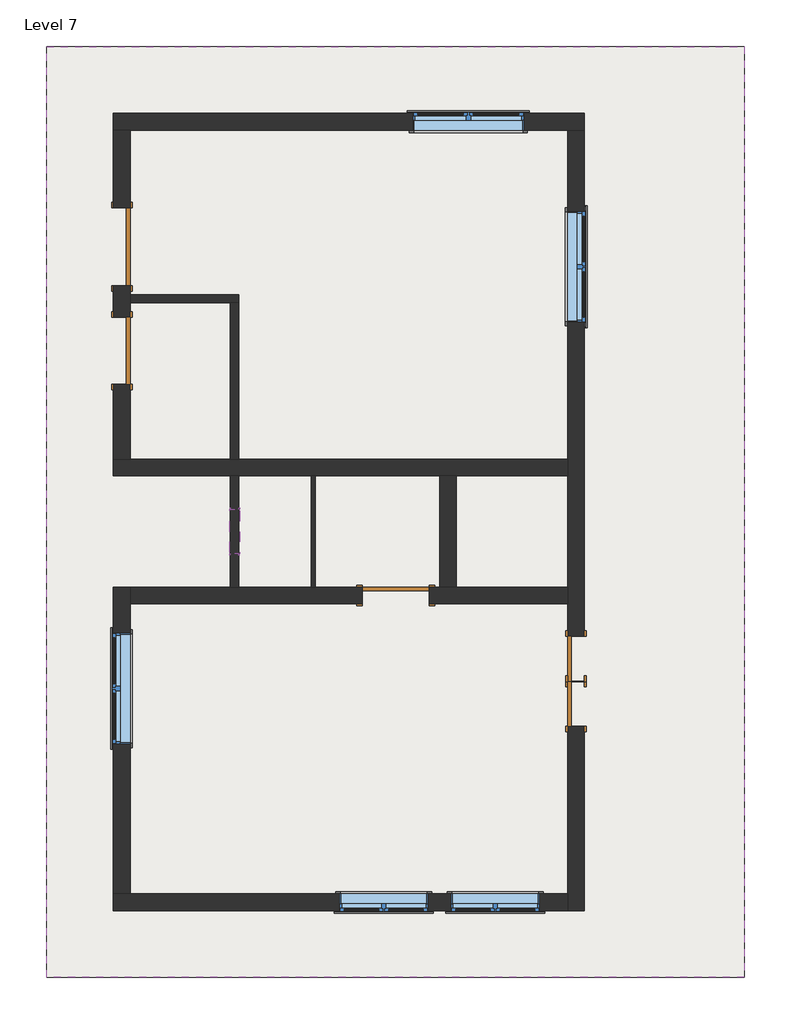
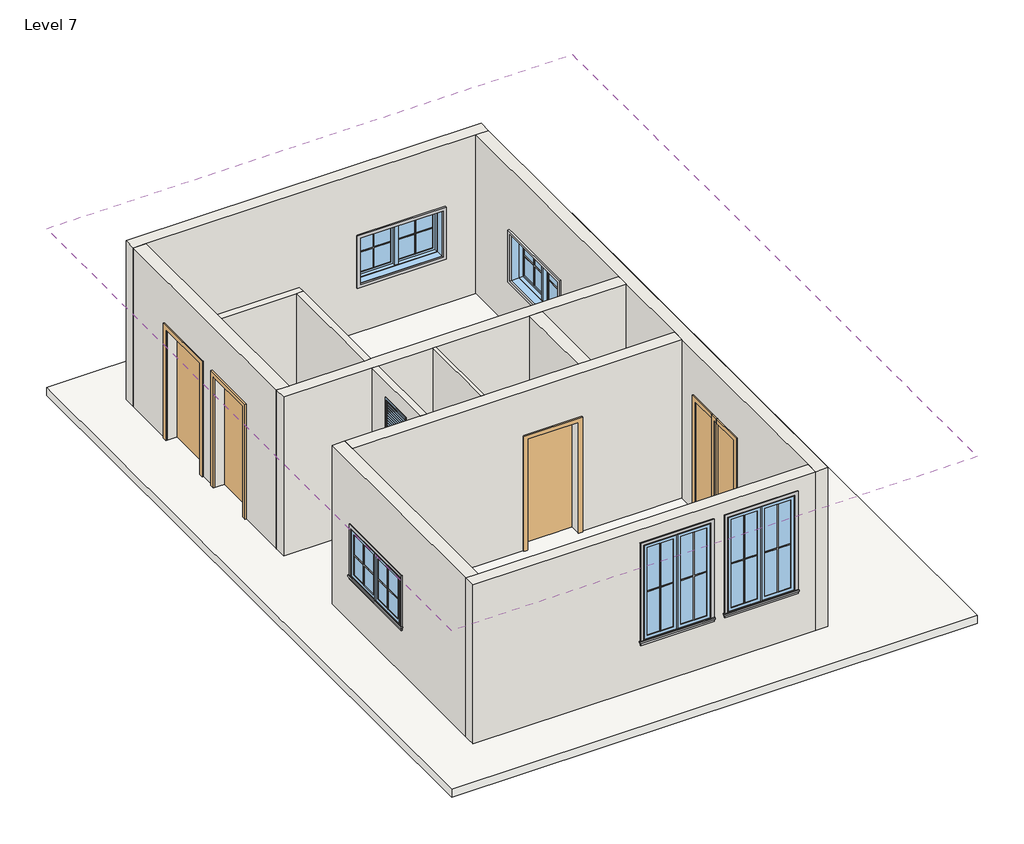
# One storey, incomplete: 20 proxies, 12 walls, 6 windows, 5 doors, 2 roofs.
"""IFC4 building model written with IfcOpenShell, lengths in millimetres."""

from ifc_helpers import new_model, si_unit, frame, origin, place, context, project, spatial, polyline, outline, extrude, faceted_brep, transform, mapped, element, save
from components import muntin_pattern_2x2_muntin_pattern_2x2_9352d081, muntin_pattern_2x2_muntin_pattern_2x2_5c2cbe28, muntin_pattern_2x2_muntin_pattern_2x2_2b4d9f72, muntin_pattern_2x2_muntin_pattern_2x2_ef995ed3, trim_window_exterior_flat_with_sill_979bde60, trim_window_exterior_flat_with_sill_b7e4d11c, trim_window_interior_flat_picture_frame_7883d11b, trim_window_interior_flat_picture_frame_936b8d2a, single_flush_door_2_0d3b4037, single_flush_door_2_4a3212df, door_a90ba1ad, door_0ca8825f, door_9d399b00, window_casement_double_c1d95f0f, window_casement_double_wall_4_6ca1769e, window_d39e7ecb

model = new_model("IFC4")

# Units and contexts
model_context = context("Model", 3, world=origin())
ifc_project = project(units=[si_unit("LENGTHUNIT", "METRE", prefix="MILLI")], contexts=[model_context])

# Site, building, storey
site = spatial("IfcSite", under=ifc_project)
building = spatial("IfcBuilding", under=site)
storey = spatial("IfcBuildingStorey", under=building, Name="Level 7", Elevation=16002.0)

# Proxies
placement = place(None, origin())
muntin_pattern_2x2_muntin_pattern_2x2_shape = muntin_pattern_2x2_muntin_pattern_2x2_9352d081(model_context)
element("IfcBuildingElementProxy", 1, Name="Muntin Pattern_2x2 : Muntin Pattern_2x2", ObjectType="Muntin Pattern_2x2 : Muntin Pattern_2x2", at=placement, inside=storey, context=model_context, shape_type="MappedRepresentation", body=[
    mapped(muntin_pattern_2x2_muntin_pattern_2x2_shape, transform((-4785.3510342, -2707.8617544, 16986.25), x_axis=(0.0, 1.0, 0.0), y_axis=(-1.0, 0.0, 0.0), z_axis=(0.0, 0.0, 1.0))),
])
element("IfcBuildingElementProxy", 2, Name="Muntin Pattern_2x2 : Muntin Pattern_2x2", ObjectType="Muntin Pattern_2x2 : Muntin Pattern_2x2", at=placement, inside=storey, context=model_context, shape_type="MappedRepresentation", body=[
    mapped(muntin_pattern_2x2_muntin_pattern_2x2_shape, transform((1634.4989658, 3816.7632456, 16986.25), x_axis=(0.0, -1.0, 0.0), y_axis=(1.0, 0.0, 0.0), z_axis=(0.0, 0.0, 1.0))),
])
element("IfcBuildingElementProxy", 3, Name="Muntin Pattern_2x2 : Muntin Pattern_2x2", ObjectType="Muntin Pattern_2x2 : Muntin Pattern_2x2", at=placement, inside=storey, context=model_context, shape_type="MappedRepresentation", body=[
    mapped(muntin_pattern_2x2_muntin_pattern_2x2_shape, transform((-322.8885342, 5523.3257456, 16986.25), x_axis=(1.0, 0.0, 0.0), y_axis=(0.0, 1.0, 0.0), z_axis=(0.0, 0.0, 1.0))),
])
muntin_pattern_2x2_muntin_pattern_2x2_2_shape = muntin_pattern_2x2_muntin_pattern_2x2_5c2cbe28(model_context)
element("IfcBuildingElementProxy", 4, Name="Muntin Pattern_2x2 : Muntin Pattern_2x2", ObjectType="Muntin Pattern_2x2 : Muntin Pattern_2x2", at=placement, inside=storey, context=model_context, shape_type="MappedRepresentation", body=[
    mapped(muntin_pattern_2x2_muntin_pattern_2x2_2_shape, transform((-4785.3510342, -1949.0367544, 16986.25), x_axis=(0.0, -1.0, 0.0), y_axis=(1.0, 0.0, 0.0), z_axis=(0.0, 0.0, 1.0))),
])
element("IfcBuildingElementProxy", 5, Name="Muntin Pattern_2x2 : Muntin Pattern_2x2", ObjectType="Muntin Pattern_2x2 : Muntin Pattern_2x2", at=placement, inside=storey, context=model_context, shape_type="MappedRepresentation", body=[
    mapped(muntin_pattern_2x2_muntin_pattern_2x2_2_shape, transform((1634.4989658, 3057.9382456, 16986.25), x_axis=(0.0, 1.0, 0.0), y_axis=(-1.0, 0.0, 0.0), z_axis=(0.0, 0.0, 1.0))),
])
element("IfcBuildingElementProxy", 6, Name="Muntin Pattern_2x2 : Muntin Pattern_2x2", ObjectType="Muntin Pattern_2x2 : Muntin Pattern_2x2", at=placement, inside=storey, context=model_context, shape_type="MappedRepresentation", body=[
    mapped(muntin_pattern_2x2_muntin_pattern_2x2_2_shape, transform((435.9364658, 5523.3257456, 16986.25), x_axis=(-1.0, 0.0, 0.0), y_axis=(0.0, -1.0, 0.0), z_axis=(0.0, 0.0, 1.0))),
])
muntin_pattern_2x2_muntin_pattern_2x2_3_shape = muntin_pattern_2x2_muntin_pattern_2x2_2b4d9f72(model_context)
element("IfcBuildingElementProxy", 7, Name="Muntin Pattern_2x2 : Muntin Pattern_2x2", ObjectType="Muntin Pattern_2x2 : Muntin Pattern_2x2", at=placement, inside=storey, context=model_context, shape_type="MappedRepresentation", body=[
    mapped(muntin_pattern_2x2_muntin_pattern_2x2_3_shape, transform((-795.9635342, -5354.2242544, 16986.25), x_axis=(-1.0, 0.0, 0.0), y_axis=(0.0, -1.0, 0.0), z_axis=(0.0, 0.0, 1.0))),
])
element("IfcBuildingElementProxy", 8, Name="Muntin Pattern_2x2 : Muntin Pattern_2x2", ObjectType="Muntin Pattern_2x2 : Muntin Pattern_2x2", at=placement, inside=storey, context=model_context, shape_type="MappedRepresentation", body=[
    mapped(muntin_pattern_2x2_muntin_pattern_2x2_3_shape, transform((728.0364658, -5354.2242544, 16986.25), x_axis=(-1.0, 0.0, 0.0), y_axis=(0.0, -1.0, 0.0), z_axis=(0.0, 0.0, 1.0))),
])
muntin_pattern_2x2_muntin_pattern_2x2_4_shape = muntin_pattern_2x2_muntin_pattern_2x2_ef995ed3(model_context)
element("IfcBuildingElementProxy", 9, Name="Muntin Pattern_2x2 : Muntin Pattern_2x2", ObjectType="Muntin Pattern_2x2 : Muntin Pattern_2x2", at=placement, inside=storey, context=model_context, shape_type="MappedRepresentation", body=[
    mapped(muntin_pattern_2x2_muntin_pattern_2x2_4_shape, transform((-1402.3885342, -5354.2242544, 16986.25), x_axis=(1.0, 0.0, 0.0), y_axis=(0.0, 1.0, 0.0), z_axis=(0.0, 0.0, 1.0))),
])
element("IfcBuildingElementProxy", 10, Name="Muntin Pattern_2x2 : Muntin Pattern_2x2", ObjectType="Muntin Pattern_2x2 : Muntin Pattern_2x2", at=placement, inside=storey, context=model_context, shape_type="MappedRepresentation", body=[
    mapped(muntin_pattern_2x2_muntin_pattern_2x2_4_shape, transform((121.6114658, -5354.2242544, 16986.25), x_axis=(1.0, 0.0, 0.0), y_axis=(0.0, 1.0, 0.0), z_axis=(0.0, 0.0, 1.0))),
])
trim_window_exterior_flat_with_sill_shape = trim_window_exterior_flat_with_sill_979bde60(model_context)
element("IfcBuildingElementProxy", 11, Name="Trim-Window-Exterior-Flat : with Sill", ObjectType="Trim-Window-Exterior-Flat : with Sill", at=placement, inside=storey, context=model_context, shape_type="MappedRepresentation", body=[
    mapped(trim_window_exterior_flat_with_sill_shape, transform((-4794.8760342, -2328.4492544, 17830.8), x_axis=(0.0, -1.0, 0.0), y_axis=(0.0, 0.0, 1.0), z_axis=(-1.0, 0.0, 0.0))),
])
element("IfcBuildingElementProxy", 12, Name="Trim-Window-Exterior-Flat : with Sill", ObjectType="Trim-Window-Exterior-Flat : with Sill", at=placement, inside=storey, context=model_context, shape_type="MappedRepresentation", body=[
    mapped(trim_window_exterior_flat_with_sill_shape, transform((1644.0239658, 3437.3507456, 17830.8), x_axis=(0.0, 1.0, 0.0), y_axis=(0.0, 0.0, 1.0), z_axis=(1.0, 0.0, 0.0))),
])
element("IfcBuildingElementProxy", 13, Name="Trim-Window-Exterior-Flat : with Sill", ObjectType="Trim-Window-Exterior-Flat : with Sill", at=placement, inside=storey, context=model_context, shape_type="MappedRepresentation", body=[
    mapped(trim_window_exterior_flat_with_sill_shape, transform((56.5239658, 5532.8507456, 17830.8), x_axis=(-1.0, 0.0, 0.0), y_axis=(0.0, 0.0, 1.0), z_axis=(0.0, 1.0, 0.0))),
])
trim_window_exterior_flat_with_sill_2_shape = trim_window_exterior_flat_with_sill_b7e4d11c(model_context)
element("IfcBuildingElementProxy", 14, Name="Trim-Window-Exterior-Flat : with Sill", ObjectType="Trim-Window-Exterior-Flat : with Sill", at=placement, inside=storey, context=model_context, shape_type="MappedRepresentation", body=[
    mapped(trim_window_exterior_flat_with_sill_2_shape, transform((-1099.1760342, -5363.7492544, 18745.2), x_axis=(1.0, 0.0, 0.0), y_axis=(0.0, 0.0, 1.0), z_axis=(0.0, -1.0, 0.0))),
])
element("IfcBuildingElementProxy", 15, Name="Trim-Window-Exterior-Flat : with Sill", ObjectType="Trim-Window-Exterior-Flat : with Sill", at=placement, inside=storey, context=model_context, shape_type="MappedRepresentation", body=[
    mapped(trim_window_exterior_flat_with_sill_2_shape, transform((424.8239658, -5363.7492544, 18745.2), x_axis=(1.0, 0.0, 0.0), y_axis=(0.0, 0.0, 1.0), z_axis=(0.0, -1.0, 0.0))),
])
trim_window_interior_flat_picture_frame_shape = trim_window_interior_flat_picture_frame_7883d11b(model_context)
element("IfcBuildingElementProxy", 16, Name="Trim-Window-Interior-Flat : Picture Frame", ObjectType="Trim-Window-Interior-Flat : Picture Frame", at=placement, inside=storey, context=model_context, shape_type="MappedRepresentation", body=[
    mapped(trim_window_interior_flat_picture_frame_shape, transform((-4566.2760342, -2328.4492544, 17830.8), x_axis=(0.0, 1.0, 0.0), y_axis=(0.0, 0.0, 1.0), z_axis=(1.0, 0.0, 0.0))),
])
element("IfcBuildingElementProxy", 17, Name="Trim-Window-Interior-Flat : Picture Frame", ObjectType="Trim-Window-Interior-Flat : Picture Frame", at=placement, inside=storey, context=model_context, shape_type="MappedRepresentation", body=[
    mapped(trim_window_interior_flat_picture_frame_shape, transform((1415.4239658, 3437.3507456, 17830.8), x_axis=(0.0, -1.0, 0.0), y_axis=(0.0, 0.0, 1.0), z_axis=(-1.0, 0.0, 0.0))),
])
element("IfcBuildingElementProxy", 18, Name="Trim-Window-Interior-Flat : Picture Frame", ObjectType="Trim-Window-Interior-Flat : Picture Frame", at=placement, inside=storey, context=model_context, shape_type="MappedRepresentation", body=[
    mapped(trim_window_interior_flat_picture_frame_shape, transform((56.5239658, 5304.2507456, 17830.8), x_axis=(1.0, 0.0, 0.0), y_axis=(0.0, 0.0, 1.0), z_axis=(0.0, -1.0, 0.0))),
])
trim_window_interior_flat_picture_frame_2_shape = trim_window_interior_flat_picture_frame_936b8d2a(model_context)
element("IfcBuildingElementProxy", 19, Name="Trim-Window-Interior-Flat : Picture Frame", ObjectType="Trim-Window-Interior-Flat : Picture Frame", at=placement, inside=storey, context=model_context, shape_type="MappedRepresentation", body=[
    mapped(trim_window_interior_flat_picture_frame_2_shape, transform((-1099.1760342, -5135.1492544, 18745.2), x_axis=(-1.0, 0.0, 0.0), y_axis=(0.0, 0.0, 1.0), z_axis=(0.0, 1.0, 0.0))),
])
element("IfcBuildingElementProxy", 20, Name="Trim-Window-Interior-Flat : Picture Frame", ObjectType="Trim-Window-Interior-Flat : Picture Frame", at=placement, inside=storey, context=model_context, shape_type="MappedRepresentation", body=[
    mapped(trim_window_interior_flat_picture_frame_2_shape, transform((424.8239658, -5135.1492544, 18745.2), x_axis=(-1.0, 0.0, 0.0), y_axis=(0.0, 0.0, 1.0), z_axis=(0.0, 1.0, 0.0))),
])

# Doors
single_flush_door_2_shape = single_flush_door_2_0d3b4037(model_context)
element("IfcDoor", 21, ObjectType="Single-Flush : door 2'", at=placement, inside=storey, context=model_context, shape_type="MappedRepresentation", body=[
    mapped(single_flush_door_2_shape, transform((1529.7239658, -1922.0492544, 16002.0), x_axis=(0.0, 1.0, 0.0), y_axis=(-1.0, 0.0, 0.0), z_axis=(0.0, 0.0, 1.0))),
])
single_flush_door_2_2_shape = single_flush_door_2_4a3212df(model_context)
element("IfcDoor", 22, ObjectType="Single-Flush : door 2'", at=placement, inside=storey, context=model_context, shape_type="MappedRepresentation", body=[
    mapped(single_flush_door_2_2_shape, transform((1529.7239658, -2537.9992544, 16002.0), x_axis=(0.0, -1.0, 0.0), y_axis=(1.0, 0.0, 0.0), z_axis=(0.0, 0.0, 1.0))),
])
door_shape = door_a90ba1ad(model_context)
element("IfcDoor", 23, ObjectType="Single-Flush : door 2'6\"", at=placement, inside=storey, context=model_context, shape_type="MappedRepresentation", body=[
    mapped(door_shape, transform((-4680.5760342, 2288.0007456, 16002.0), x_axis=(0.0, 1.0, 0.0), y_axis=(-1.0, 0.0, 0.0), z_axis=(0.0, 0.0, 1.0))),
])
door_2_shape = door_0ca8825f(model_context)
element("IfcDoor", 24, ObjectType="Single-Flush : door 2'6\"", at=placement, inside=storey, context=model_context, shape_type="MappedRepresentation", body=[
    mapped(door_2_shape, transform((-934.0760342, -1058.4492544, 16002.0), x_axis=(1.0, 0.0, 0.0), y_axis=(0.0, 1.0, 0.0), z_axis=(0.0, 0.0, 1.0))),
])
door_3_shape = door_9d399b00(model_context)
element("IfcDoor", 25, ObjectType="Single-Flush : door 3'6\"", at=placement, inside=storey, context=model_context, shape_type="MappedRepresentation", body=[
    mapped(door_3_shape, transform((-4680.5760342, 3710.4007456, 16002.0), x_axis=(0.0, -1.0, 0.0), y_axis=(1.0, 0.0, 0.0), z_axis=(0.0, 0.0, 1.0))),
])

# Roofs
element("IfcRoof", 26, ObjectType="roof 6\"", at=placement, inside=storey, context=model_context, shape_type="SweptSolid", body=[
    extrude(outline(polyline([(-5709.2760342, 6447.2507456), (3828.4239658, 6447.2507456), (3828.4239658, -6278.1492544), (-5709.2760342, -6278.1492544), (-5709.2760342, 6447.2507456)])), frame((0.0, 0.0, 15849.6), z_axis=(0.0, 0.0, 1.0), x_axis=(1.0, 0.0, 0.0)), (0.0, 0.0, 1.0), 152.4),
])
element("IfcRoof", 27, ObjectType="roof 6\"", at=placement, inside=storey, context=model_context, shape_type="SweptSolid", body=[
    extrude(outline(polyline([(-5709.2760342, 6447.2507456), (3828.4239658, 6447.2507456), (3828.4239658, -6278.1492544), (-5709.2760342, -6278.1492544), (-5709.2760342, 6447.2507456)])), frame((0.0, 0.0, 19050.0), z_axis=(0.0, 0.0, 1.0), x_axis=(1.0, 0.0, 0.0)), (0.0, 0.0, 1.0), 152.4),
])

# Walls
element("IfcWall", 28, ObjectType="wall 2\"", at=placement, inside=storey, context=model_context, shape_type="SweptSolid", body=[
    extrude(outline(polyline([(-2089.7760342, -944.1492544), (-2089.7760342, 579.8507456), (-2038.9760342, 579.8507456), (-2038.9760342, -944.1492544), (-2089.7760342, -944.1492544)])), frame((0.0, 0.0, 16002.0), z_axis=(0.0, 0.0, 1.0), x_axis=(1.0, 0.0, 0.0)), (0.0, 0.0, 1.0), 3048.0),
])
element("IfcWall", 29, ObjectType="wall 4.5\"", at=placement, inside=storey, context=model_context, shape_type="Brep", body=[
    faceted_brep([(-4566.2760342, 2942.0507456, 16002.0), (-3194.6760342, 2942.0507456, 16002.0), (-3080.3760342, 2942.0507456, 16002.0), (-3080.3760342, 2942.0507456, 19050.0), (-3194.6760342, 2942.0507456, 19050.0), (-4566.2760342, 2942.0507456, 19050.0), (-4566.2760342, 3056.3507456, 16002.0), (-4566.2760342, 3056.3507456, 19050.0), (-3080.3760342, 3056.3507456, 19050.0), (-3080.3760342, 3056.3507456, 16002.0)], [[[0, 1, 2, 3, 4, 5]], [[6, 7, 8, 9]], [[2, 1, 0, 6, 9]], [[0, 5, 7, 6]], [[3, 2, 9, 8]], [[5, 4, 3, 8, 7]]]),
])
element("IfcWall", 30, ObjectType="wall 4.5\"", at=placement, inside=storey, context=model_context, shape_type="SweptSolid", body=[
    extrude(outline(polyline([(-3194.6760342, 808.4507456), (-3194.6760342, 2942.0507456), (-3080.3760342, 2942.0507456), (-3080.3760342, 808.4507456), (-3194.6760342, 808.4507456)])), frame((0.0, 0.0, 16002.0), z_axis=(0.0, 0.0, 1.0), x_axis=(1.0, 0.0, 0.0)), (0.0, 0.0, 1.0), 3048.0),
])
element("IfcWall", 31, ObjectType="wall 4.5\"", at=placement, inside=storey, context=model_context, shape_type="SweptSolid", body=[
    extrude(outline(polyline([(579.8507456, 16002.0), (-944.1492544, 16002.0), (-944.1492544, 19050.0), (579.8507456, 19050.0), (579.8507456, 16002.0)]), holes=[polyline([(-486.9492544, 18745.2), (-486.9492544, 18135.6), (122.6507456, 18135.6), (122.6507456, 18745.2), (-486.9492544, 18745.2)])]), frame((-3194.6760342, 0.0, 0.0), z_axis=(1.0, 0.0, 0.0), x_axis=(0.0, 1.0, 0.0)), (0.0, 0.0, 1.0), 114.3),
])
element("IfcWall", 32, ObjectType="wall 9\"", at=placement, inside=storey, context=model_context, shape_type="Brep", body=[
    faceted_brep([(-4794.8760342, 5304.2507456, 16002.0), (-4566.2760342, 5304.2507456, 16002.0), (1415.4239658, 5304.2507456, 16002.0), (1644.0239658, 5304.2507456, 16002.0), (1644.0239658, 5304.2507456, 19050.0), (1415.4239658, 5304.2507456, 19050.0), (-4566.2760342, 5304.2507456, 19050.0), (-4794.8760342, 5304.2507456, 19050.0), (818.5239658, 5304.2507456, 17830.8), (818.5239658, 5304.2507456, 16916.4), (-705.4760342, 5304.2507456, 16916.4), (-705.4760342, 5304.2507456, 17830.8), (-4794.8760342, 5532.8507456, 16002.0), (-4794.8760342, 5532.8507456, 19050.0), (1644.0239658, 5532.8507456, 19050.0), (1644.0239658, 5532.8507456, 16002.0), (818.5239658, 5532.8507456, 17830.8), (-705.4760342, 5532.8507456, 17830.8), (-705.4760342, 5532.8507456, 16916.4), (818.5239658, 5532.8507456, 16916.4)], [[[0, 1, 2, 3, 4, 5, 6, 7], [8, 9, 10, 11]], [[12, 13, 14, 15], [16, 17, 18, 19]], [[3, 2, 1, 0, 12, 15]], [[4, 3, 15, 14]], [[0, 7, 13, 12]], [[9, 8, 16, 19]], [[10, 9, 19, 18]], [[11, 10, 18, 17]], [[8, 11, 17, 16]], [[7, 6, 5, 4, 14, 13]]]),
])
element("IfcWall", 33, ObjectType="wall 9\"", at=placement, inside=storey, context=model_context, shape_type="Brep", body=[
    faceted_brep([(1415.4239658, 5304.2507456, 19050.0), (1415.4239658, 5304.2507456, 16002.0), (1415.4239658, 808.4507456, 16002.0), (1415.4239658, 579.8507456, 16002.0), (1415.4239658, -944.1492544, 16002.0), (1415.4239658, -1172.7492544, 16002.0), (1415.4239658, -1617.2492544, 16002.0), (1415.4239658, -1617.2492544, 18135.6), (1415.4239658, -2226.8492544, 18135.6), (1415.4239658, -2226.8492544, 16002.0), (1415.4239658, -2233.1992544, 16002.0), (1415.4239658, -2233.1992544, 18135.6), (1415.4239658, -2842.7992544, 18135.6), (1415.4239658, -2842.7992544, 16002.0), (1415.4239658, -5135.1492544, 16002.0), (1415.4239658, -5363.7492544, 16002.0), (1415.4239658, -5363.7492544, 19050.0), (1415.4239658, -5135.1492544, 19050.0), (1415.4239658, -1172.7492544, 19050.0), (1415.4239658, -944.1492544, 19050.0), (1415.4239658, 579.8507456, 19050.0), (1415.4239658, 808.4507456, 19050.0), (1415.4239658, 2675.3507456, 17830.8), (1415.4239658, 2675.3507456, 16916.4), (1415.4239658, 4199.3507456, 16916.4), (1415.4239658, 4199.3507456, 17830.8), (1644.0239658, 5304.2507456, 16002.0), (1644.0239658, 5304.2507456, 19050.0), (1644.0239658, -5363.7492544, 19050.0), (1644.0239658, -5363.7492544, 16002.0), (1644.0239658, -2842.7992544, 16002.0), (1644.0239658, -2842.7992544, 18135.6), (1644.0239658, -2233.1992544, 18135.6), (1644.0239658, -2233.1992544, 16002.0), (1644.0239658, -2226.8492544, 16002.0), (1644.0239658, -2226.8492544, 18135.6), (1644.0239658, -1617.2492544, 18135.6), (1644.0239658, -1617.2492544, 16002.0), (1644.0239658, 2675.3507456, 17830.8), (1644.0239658, 4199.3507456, 17830.8), (1644.0239658, 4199.3507456, 16916.4), (1644.0239658, 2675.3507456, 16916.4)], [[[0, 1, 2, 3, 4, 5, 6, 7, 8, 9, 10, 11, 12, 13, 14, 15, 16, 17, 18, 19, 20, 21], [22, 23, 24, 25]], [[26, 27, 28, 29, 30, 31, 32, 33, 34, 35, 36, 37], [38, 39, 40, 41]], [[1, 26, 37, 6, 5, 4, 3, 2]], [[29, 15, 14, 13, 30]], [[9, 34, 33, 10]], [[1, 0, 27, 26]], [[16, 15, 29, 28]], [[23, 22, 38, 41]], [[24, 23, 41, 40]], [[25, 24, 40, 39]], [[22, 25, 39, 38]], [[7, 6, 37, 36]], [[8, 7, 36, 35]], [[9, 8, 35, 34]], [[12, 31, 30, 13]], [[31, 12, 11, 32]], [[32, 11, 10, 33]], [[0, 21, 20, 19, 18, 17, 16, 28, 27]]]),
])
element("IfcWall", 34, ObjectType="wall 9\"", at=placement, inside=storey, context=model_context, shape_type="Brep", body=[
    faceted_brep([(1415.4239658, 808.4507456, 16002.0), (-3080.3760342, 808.4507456, 16002.0), (-3194.6760342, 808.4507456, 16002.0), (-4566.2760342, 808.4507456, 16002.0), (-4794.8760342, 808.4507456, 16002.0), (-4794.8760342, 808.4507456, 19050.0), (-4566.2760342, 808.4507456, 19050.0), (-3194.6760342, 808.4507456, 19050.0), (-3080.3760342, 808.4507456, 19050.0), (1415.4239658, 808.4507456, 19050.0), (1415.4239658, 579.8507456, 16002.0), (1415.4239658, 579.8507456, 19050.0), (-108.5760342, 579.8507456, 19050.0), (-337.1760342, 579.8507456, 19050.0), (-2038.9760342, 579.8507456, 19050.0), (-2089.7760342, 579.8507456, 19050.0), (-3080.3760342, 579.8507456, 19050.0), (-3194.6760342, 579.8507456, 19050.0), (-4794.8760342, 579.8507456, 19050.0), (-4794.8760342, 579.8507456, 16002.0), (-3194.6760342, 579.8507456, 16002.0), (-3080.3760342, 579.8507456, 16002.0), (-2089.7760342, 579.8507456, 16002.0), (-2038.9760342, 579.8507456, 16002.0), (-337.1760342, 579.8507456, 16002.0), (-108.5760342, 579.8507456, 16002.0)], [[[0, 1, 2, 3, 4, 5, 6, 7, 8, 9]], [[10, 11, 12, 13, 14, 15, 16, 17, 18, 19, 20, 21, 22, 23, 24, 25]], [[4, 3, 2, 1, 0, 10, 25, 24, 23, 22, 21, 20, 19]], [[0, 9, 11, 10]], [[5, 4, 19, 18]], [[9, 8, 7, 6, 5, 18, 17, 16, 15, 14, 13, 12, 11]]]),
])
element("IfcWall", 35, ObjectType="wall 9\"", at=placement, inside=storey, context=model_context, shape_type="Brep", body=[
    faceted_brep([(-4566.2760342, 2745.2007456, 18135.6), (-4566.2760342, 2745.2007456, 16002.0), (-4566.2760342, 2942.0507456, 16002.0), (-4566.2760342, 3056.3507456, 16002.0), (-4566.2760342, 3177.0007456, 16002.0), (-4566.2760342, 3177.0007456, 18135.6), (-4566.2760342, 4243.8007456, 18135.6), (-4566.2760342, 4243.8007456, 16002.0), (-4566.2760342, 5304.2507456, 16002.0), (-4566.2760342, 5304.2507456, 19050.0), (-4566.2760342, 3056.3507456, 19050.0), (-4566.2760342, 2942.0507456, 19050.0), (-4566.2760342, 808.4507456, 19050.0), (-4566.2760342, 808.4507456, 16002.0), (-4566.2760342, 1830.8007456, 16002.0), (-4566.2760342, 1830.8007456, 18135.6), (-4794.8760342, 3177.0007456, 16002.0), (-4794.8760342, 2745.2007456, 16002.0), (-4794.8760342, 2745.2007456, 18135.6), (-4794.8760342, 1830.8007456, 18135.6), (-4794.8760342, 1830.8007456, 16002.0), (-4794.8760342, 808.4507456, 16002.0), (-4794.8760342, 808.4507456, 19050.0), (-4794.8760342, 5304.2507456, 19050.0), (-4794.8760342, 5304.2507456, 16002.0), (-4794.8760342, 4243.8007456, 16002.0), (-4794.8760342, 4243.8007456, 18135.6), (-4794.8760342, 3177.0007456, 18135.6)], [[[0, 1, 2, 3, 4, 5, 6, 7, 8, 9, 10, 11, 12, 13, 14, 15]], [[16, 17, 18, 19, 20, 21, 22, 23, 24, 25, 26, 27]], [[25, 24, 8, 7]], [[14, 13, 21, 20]], [[4, 3, 2, 1, 17, 16]], [[9, 8, 24, 23]], [[13, 12, 22, 21]], [[5, 4, 16, 27]], [[6, 5, 27, 26]], [[7, 6, 26, 25]], [[18, 17, 1, 0]], [[19, 18, 0, 15]], [[20, 19, 15, 14]], [[12, 11, 10, 9, 23, 22]]]),
])
element("IfcWall", 36, ObjectType="wall 9\"", at=placement, inside=storey, context=model_context, shape_type="Brep", body=[
    faceted_brep([(1415.4239658, -5135.1492544, 16002.0), (-4566.2760342, -5135.1492544, 16002.0), (-4794.8760342, -5135.1492544, 16002.0), (-4794.8760342, -5135.1492544, 19050.0), (-4566.2760342, -5135.1492544, 19050.0), (1415.4239658, -5135.1492544, 19050.0), (-1708.7760342, -5135.1492544, 18745.2), (-1708.7760342, -5135.1492544, 16916.4), (-489.5760342, -5135.1492544, 16916.4), (-489.5760342, -5135.1492544, 18745.2), (-184.7760342, -5135.1492544, 18745.2), (-184.7760342, -5135.1492544, 16916.4), (1034.4239658, -5135.1492544, 16916.4), (1034.4239658, -5135.1492544, 18745.2), (1415.4239658, -5363.7492544, 16002.0), (1415.4239658, -5363.7492544, 19050.0), (-4794.8760342, -5363.7492544, 19050.0), (-4794.8760342, -5363.7492544, 16002.0), (-1708.7760342, -5363.7492544, 18745.2), (-489.5760342, -5363.7492544, 18745.2), (-489.5760342, -5363.7492544, 16916.4), (-1708.7760342, -5363.7492544, 16916.4), (-184.7760342, -5363.7492544, 18745.2), (1034.4239658, -5363.7492544, 18745.2), (1034.4239658, -5363.7492544, 16916.4), (-184.7760342, -5363.7492544, 16916.4)], [[[0, 1, 2, 3, 4, 5], [6, 7, 8, 9], [10, 11, 12, 13]], [[14, 15, 16, 17], [18, 19, 20, 21], [22, 23, 24, 25]], [[2, 1, 0, 14, 17]], [[0, 5, 15, 14]], [[3, 2, 17, 16]], [[7, 6, 18, 21]], [[8, 7, 21, 20]], [[9, 8, 20, 19]], [[6, 9, 19, 18]], [[11, 10, 22, 25]], [[12, 11, 25, 24]], [[13, 12, 24, 23]], [[10, 13, 23, 22]], [[5, 4, 3, 16, 15]]]),
])
element("IfcWall", 37, ObjectType="wall 9\"", at=placement, inside=storey, context=model_context, shape_type="Brep", body=[
    faceted_brep([(-4566.2760342, -5135.1492544, 16002.0), (-4566.2760342, -1172.7492544, 16002.0), (-4566.2760342, -944.1492544, 16002.0), (-4566.2760342, -944.1492544, 19050.0), (-4566.2760342, -1172.7492544, 19050.0), (-4566.2760342, -5135.1492544, 19050.0), (-4566.2760342, -1566.4492544, 17830.8), (-4566.2760342, -1566.4492544, 16916.4), (-4566.2760342, -3090.4492544, 16916.4), (-4566.2760342, -3090.4492544, 17830.8), (-4794.8760342, -5135.1492544, 16002.0), (-4794.8760342, -5135.1492544, 19050.0), (-4794.8760342, -944.1492544, 19050.0), (-4794.8760342, -944.1492544, 16002.0), (-4794.8760342, -1566.4492544, 17830.8), (-4794.8760342, -3090.4492544, 17830.8), (-4794.8760342, -3090.4492544, 16916.4), (-4794.8760342, -1566.4492544, 16916.4)], [[[0, 1, 2, 3, 4, 5], [6, 7, 8, 9]], [[10, 11, 12, 13], [14, 15, 16, 17]], [[2, 1, 0, 10, 13]], [[0, 5, 11, 10]], [[3, 2, 13, 12]], [[7, 6, 14, 17]], [[8, 7, 17, 16]], [[9, 8, 16, 15]], [[6, 9, 15, 14]], [[5, 4, 3, 12, 11]]]),
])
element("IfcWall", 38, ObjectType="wall 9\"", at=placement, inside=storey, context=model_context, shape_type="Brep", body=[
    faceted_brep([(-476.8760342, -1172.7492544, 18135.6), (-476.8760342, -1172.7492544, 16002.0), (1415.4239658, -1172.7492544, 16002.0), (1415.4239658, -1172.7492544, 19050.0), (-4566.2760342, -1172.7492544, 19050.0), (-4566.2760342, -1172.7492544, 16002.0), (-1391.2760342, -1172.7492544, 16002.0), (-1391.2760342, -1172.7492544, 18135.6), (1415.4239658, -944.1492544, 16002.0), (-108.5760342, -944.1492544, 16002.0), (-337.1760342, -944.1492544, 16002.0), (-476.8760342, -944.1492544, 16002.0), (-476.8760342, -944.1492544, 18135.6), (-1391.2760342, -944.1492544, 18135.6), (-1391.2760342, -944.1492544, 16002.0), (-2038.9760342, -944.1492544, 16002.0), (-2089.7760342, -944.1492544, 16002.0), (-3080.3760342, -944.1492544, 16002.0), (-3194.6760342, -944.1492544, 16002.0), (-4566.2760342, -944.1492544, 16002.0), (-4566.2760342, -944.1492544, 19050.0), (-3194.6760342, -944.1492544, 19050.0), (-3080.3760342, -944.1492544, 19050.0), (-2089.7760342, -944.1492544, 19050.0), (-2038.9760342, -944.1492544, 19050.0), (-337.1760342, -944.1492544, 19050.0), (-108.5760342, -944.1492544, 19050.0), (1415.4239658, -944.1492544, 19050.0)], [[[0, 1, 2, 3, 4, 5, 6, 7]], [[8, 9, 10, 11, 12, 13, 14, 15, 16, 17, 18, 19, 20, 21, 22, 23, 24, 25, 26, 27]], [[6, 5, 19, 18, 17, 16, 15, 14]], [[2, 1, 11, 10, 9, 8]], [[5, 4, 20, 19]], [[3, 2, 8, 27]], [[12, 11, 1, 0]], [[13, 12, 0, 7]], [[14, 13, 7, 6]], [[4, 3, 27, 26, 25, 24, 23, 22, 21, 20]]]),
])
element("IfcWall", 39, ObjectType="wall 9\"", at=placement, inside=storey, context=model_context, shape_type="SweptSolid", body=[
    extrude(outline(polyline([(-108.5760342, 579.8507456), (-108.5760342, -944.1492544), (-337.1760342, -944.1492544), (-337.1760342, 579.8507456), (-108.5760342, 579.8507456)])), frame((0.0, 0.0, 16002.0), z_axis=(0.0, 0.0, 1.0), x_axis=(1.0, 0.0, 0.0)), (0.0, 0.0, 1.0), 3048.0),
])

# Windows
window_casement_double_shape = window_casement_double_c1d95f0f(model_context)
element("IfcWindow", 40, ObjectType="Window-Casement-Double", at=placement, inside=storey, context=model_context, shape_type="MappedRepresentation", body=[
    mapped(window_casement_double_shape, transform((-4680.5760342, -2328.4492544, 16002.0), x_axis=(0.0, 1.0, 0.0), y_axis=(-1.0, 0.0, 0.0), z_axis=(0.0, 0.0, 1.0))),
])
element("IfcWindow", 41, ObjectType="Window-Casement-Double", at=placement, inside=storey, context=model_context, shape_type="MappedRepresentation", body=[
    mapped(window_casement_double_shape, transform((1529.7239658, 3437.3507456, 16002.0), x_axis=(0.0, -1.0, 0.0), y_axis=(1.0, 0.0, 0.0), z_axis=(0.0, 0.0, 1.0))),
])
element("IfcWindow", 42, ObjectType="Window-Casement-Double", at=placement, inside=storey, context=model_context, shape_type="MappedRepresentation", body=[
    mapped(window_casement_double_shape, transform((56.5239658, 5418.5507456, 16002.0), x_axis=(1.0, 0.0, 0.0), y_axis=(0.0, 1.0, 0.0), z_axis=(0.0, 0.0, 1.0))),
])
window_casement_double_wall_4_shape = window_casement_double_wall_4_6ca1769e(model_context)
element("IfcWindow", 43, ObjectType="Window-Casement-Double : wall 4'", at=placement, inside=storey, context=model_context, shape_type="MappedRepresentation", body=[
    mapped(window_casement_double_wall_4_shape, transform((-1099.1760342, -5249.4492544, 16002.0), x_axis=(-1.0, 0.0, 0.0), y_axis=(0.0, -1.0, 0.0), z_axis=(0.0, 0.0, 1.0))),
])
element("IfcWindow", 44, ObjectType="Window-Casement-Double : wall 4'", at=placement, inside=storey, context=model_context, shape_type="MappedRepresentation", body=[
    mapped(window_casement_double_wall_4_shape, transform((424.8239658, -5249.4492544, 16002.0), x_axis=(-1.0, 0.0, 0.0), y_axis=(0.0, -1.0, 0.0), z_axis=(0.0, 0.0, 1.0))),
])
window_shape = window_d39e7ecb(model_context)
element("IfcWindow", 45, ObjectType="Window-Louvers : 24\" x 24\"", at=placement, inside=storey, context=model_context, shape_type="MappedRepresentation", body=[
    mapped(window_shape, transform((-3143.8760342, -182.1492544, 17221.2), x_axis=(0.0, 1.0, 0.0), y_axis=(-1.0, 0.0, 0.0), z_axis=(0.0, 0.0, 1.0))),
])

save(model, "model.ifc")

# Revit data of these elements
# Type "Muntin Pattern_2x2 : Muntin Pattern_2x2"
#   Width [instance default] = 4' - 0"
#   Thickness = 0' - 0 1/2"
#   Height [instance default] = 4' - 0"
#   Distance = 0' - 0 3/4"
#   Interior Material [instance default] = none
#   Exterior Material [instance default] = none
#   Default Elevation = 0
# Type "Trim-Window-Exterior-Flat : with Sill"
#   Trim Width = 0' - 2 1/4"
#   Trim Thickness_Picture Frame = 0' - 1 1/4"
#   Trim Thickness_with Sill = 0' - 0 3/4"
#   Sill Thickness = 0' - 1 1/4"
#   Opening Width [instance default] = 2' - 0"
#   Opening Height [instance default] = 3' - 0"
#   Default Elevation = 4' - 0"
#   Sill = yes
#   Picture Frame = no
#   Trim Material [instance default] = none
# Type "Trim-Window-Interior-Flat : Picture Frame"
#   Trim Thickness_Picture Frame = 0' - 1 1/4"
#   Trim Width = 0' - 2 1/4"
#   Trim Thickness_with Sill = 0' - 0 3/4"
#   Sill Thickness = 0' - 1 1/4"
#   Opening Width [instance default] = 2' - 0"
#   Opening Height [instance default] = 3' - 0"
#   Default Elevation = 4' - 0"
#   Sill = no
#   Picture Frame = yes
#   Trim Material [instance default] = none
# Type "Single-Flush : door 2'"
#   Type Mark = "11"
#   Construction Type Id = "MDOOR"
#   Assembly Code = "C1020"
#   Analytic Construction = "Metal"
#   Thickness = 0' - 2"
#   Heat Transfer Coefficient (U) = 0.651978 BTU/(h·ft²·°F)
#   Height = 7' - 0"
#   Trim Projection Ext = 0' - 1"
#   Trim Projection Int = 0' - 1"
#   Trim Width = 0' - 3"
#   Width = 2' - 0"
#   Define Thermal Properties by = 1
#   Door Material = Door - Panel
#   Frame Material = Door - Frame
#   Visual Light Transmittance = 0
#   Solar Heat Gain Coefficient = 0
#   Function = (empty or 0)
#   Wall Closure = (empty or 0)
# Type "Single-Flush : door 2'6\""
#   Type Mark = "8"
#   Construction Type Id = "MDOOR"
#   Assembly Code = "C1020"
#   Analytic Construction = "Metal"
#   Thickness = 0' - 2"
#   Heat Transfer Coefficient (U) = 0.651978 BTU/(h·ft²·°F)
#   Height = 7' - 0"
#   Trim Projection Ext = 0' - 1"
#   Trim Projection Int = 0' - 1"
#   Trim Width = 0' - 3"
#   Width = 3' - 0"
#   Define Thermal Properties by = 1
#   Door Material = Door - Panel
#   Frame Material = Door - Frame
#   Visual Light Transmittance = 0
#   Solar Heat Gain Coefficient = 0
#   Function = (empty or 0)
#   Wall Closure = (empty or 0)
# Type "Single-Flush : door 3'6\""
#   Type Mark = "10"
#   Construction Type Id = "MDOOR"
#   Assembly Code = "C1020"
#   Analytic Construction = "Metal"
#   Thickness = 0' - 2"
#   Heat Transfer Coefficient (U) = 0.651978 BTU/(h·ft²·°F)
#   Height = 7' - 0"
#   Trim Projection Ext = 0' - 1"
#   Trim Projection Int = 0' - 1"
#   Trim Width = 0' - 3"
#   Width = 3' - 6"
#   Define Thermal Properties by = 1
#   Door Material = Door - Panel
#   Frame Material = Door - Frame
#   Visual Light Transmittance = 0
#   Solar Heat Gain Coefficient = 0
#   Function = (empty or 0)
#   Wall Closure = (empty or 0)
# Type "roof 6\""
#   Assembly Code = "B1020"
#   Layers, outside or top first: 0' - 6" no material (function 1)
# Type "wall 2\""
#   Assembly Code = "B2010"
#   Layers, outside or top first: 0' - 2" no material (function 1)
# Type "wall 4.5\""
#   Assembly Code = "B2010"
#   Layers, outside or top first: 0' - 4 1/2" no material (function 1)
# Type "wall 9\""
#   Assembly Code = "B2010"
#   Layers, outside or top first: 0' - 9" no material (function 1)
# Type "Window-Casement-Double"
#   Type Mark = "18"
#   Fire Rating = "0.5h"
#   Assembly Code = "B2020100"
#   Analytic Construction = "Double glazing - domestic"
#   Frame Extension [instance default] = 0' - 0 1/4"
#   Window Inset [instance default] = 0' - 0"
#   Wall Thickness [instance default] = 0' - 6"
#   Interior Wall Closure [instance default] = 0' - 2 1/4"
#   Half Width = 2' - 6"
#   Visual Light Transmittance = 0.81
#   Thermal Resistance (R) = 1.8146 (h·ft²·°F)/BTU
#   Solar Heat Gain Coefficient = 0.76
#   Rough Width = 5' - 0 1/2"
#   Rough Height = 3' - 0 1/2"
#   Height = 3' - 0"
#   Heat Transfer Coefficient (U) = 0.5511 BTU/(h·ft²·°F)
#   Exterior Wall Closure [instance default] = 0' - 1 1/4"
#   Extension Jamb [instance default] = 0' - 2 1/4"
#   Default Sill Height = 3' - 0"
#   Width = 5' - 0"
#   Muntin Visibility = yes
#   Interior Trim Visibility [instance default] = yes
#   Exterior Trim Visibility [instance default] = yes
#   Extension Jamb Visibility [instance default] = yes
#   Interior Trim Material = Wood - Stained
#   Muntin Pattern = Muntin Pattern_2x2 : Muntin Pattern_2x2
#   Interior Trim = Trim-Window-Interior-Flat : Picture Frame
#   Interior Frame Material = Wood - Stained
#   Glass Panel Material = Glass
#   Exterior Trim Material = Clad - White
#   Exterior Trim = Trim-Window-Exterior-Flat : with Sill
#   Exterior Frame Material = Clad - White
#   Wall Closure = (empty or 0)
# Type "Window-Casement-Double : wall 4'"
#   Type Mark = "19"
#   Fire Rating = "0.5h"
#   Assembly Code = "B2020100"
#   Analytic Construction = "Double glazing - domestic"
#   Frame Extension [instance default] = 0' - 0 1/4"
#   Window Inset [instance default] = 0' - 0"
#   Wall Thickness [instance default] = 0' - 6"
#   Interior Wall Closure [instance default] = 0' - 2 1/4"
#   Half Width = 2' - 0"
#   Visual Light Transmittance = 0.81
#   Thermal Resistance (R) = 1.8146 (h·ft²·°F)/BTU
#   Solar Heat Gain Coefficient = 0.76
#   Rough Width = 4' - 0 1/2"
#   Rough Height = 6' - 0 1/2"
#   Height = 6' - 0"
#   Heat Transfer Coefficient (U) = 0.5511 BTU/(h·ft²·°F)
#   Exterior Wall Closure [instance default] = 0' - 1 1/4"
#   Extension Jamb [instance default] = 0' - 2 1/4"
#   Default Sill Height = 3' - 0"
#   Width = 4' - 0"
#   Muntin Visibility = yes
#   Interior Trim Visibility [instance default] = yes
#   Exterior Trim Visibility [instance default] = yes
#   Extension Jamb Visibility [instance default] = yes
#   Interior Trim Material = Wood - Stained
#   Muntin Pattern = Muntin Pattern_2x2 : Muntin Pattern_2x2
#   Interior Trim = Trim-Window-Interior-Flat : Picture Frame
#   Interior Frame Material = Wood - Stained
#   Glass Panel Material = Glass
#   Exterior Trim Material = Clad - White
#   Exterior Trim = Trim-Window-Exterior-Flat : with Sill
#   Exterior Frame Material = Clad - White
#   Wall Closure = (empty or 0)
# Type "Window-Louvers : 24\" x 24\""
#   Type Mark = "20"
#   Construction Type Id = "GSP4R"
#   Assembly Code = "B20"
#   Analytic Construction = "1/8 in Pilkington single glazing"
#   Visual Light Transmittance = 0.9
#   Thermal Resistance (R) = 1.53941 (h·ft²·°F)/BTU
#   Solar Heat Gain Coefficient = 0.78
#   Max Height = 1' - 11.74264"
#   Height = 2' - 0"
#   Heat Transfer Coefficient (U) = 0.6496 BTU/(h·ft²·°F)
#   Blade Width [instance default] = 1' - 10 1/2"
#   Blade Vertical Thickness = 0' - 0.35355"
#   Blade Thickness = 0' - 0 1/4"
#   Blade Spacing = 0' - 1 1/2"
#   Blade Height = 0' - 1.85355"
#   Blade Depth = 0' - 3"
#   Blade Angle = 45.00°
#   Default Sill Height = 3' - 0"
#   Trim Projection_Exterior = 0' - 0 1/2"
#   Trim Projection_Interior = 0' - 0 1/2"
#   Trim Width_Exterior = 0' - 1 1/2"
#   Trim Width_Interior = 0' - 1 1/2"
#   Width = 2' - 0"
#   Max Blade Count = 12
#   Define Thermal Properties by = 1
#   Blade Count = 12
#   Frame Material = Birch
#   Louver Material = Birch
#   Trim Exterior Material = Birch
#   Trim Interior Material = Birch
#   Wall Closure = (empty or 0)
# Elements 1, 2, 3, 4, 5, 6 (IfcBuildingElementProxy, "Muntin Pattern_2x2 : Muntin Pattern_2x2")
#   Width = 2' - 0 5/8"
#   Height = 2' - 6 1/2"
#   Interior Material = Wood - Stained
#   Exterior Material = Clad - White
#   Phase Created = New Construction
#   Materials on its faces: "Clad - White", "Wood - Stained"
# Elements 7, 8, 9, 10 (IfcBuildingElementProxy, "Muntin Pattern_2x2 : Muntin Pattern_2x2")
#   Width = 1' - 6 5/8"
#   Height = 5' - 6 1/2"
#   Interior Material = Wood - Stained
#   Exterior Material = Clad - White
#   Phase Created = New Construction
#   Materials on its faces: "Clad - White", "Wood - Stained"
# Elements 11, 12, 13 (IfcBuildingElementProxy, "Trim-Window-Exterior-Flat : with Sill")
#   Opening Width = 5' - 0"
#   Opening Height = 3' - 0"
#   Trim Material = Clad - White
#   Phase Created = New Construction
#   Materials on its faces: "Clad - White"
# Elements 14, 15 (IfcBuildingElementProxy, "Trim-Window-Exterior-Flat : with Sill")
#   Opening Width = 4' - 0"
#   Opening Height = 6' - 0"
#   Trim Material = Clad - White
#   Phase Created = New Construction
#   Materials on its faces: "Clad - White"
# Elements 16, 17, 18 (IfcBuildingElementProxy, "Trim-Window-Interior-Flat : Picture Frame")
#   Opening Width = 5' - 0"
#   Opening Height = 3' - 0"
#   Trim Material = Wood - Stained
#   Phase Created = New Construction
#   Materials on its faces: "Wood - Stained"
# Elements 19, 20 (IfcBuildingElementProxy, "Trim-Window-Interior-Flat : Picture Frame")
#   Opening Width = 4' - 0"
#   Opening Height = 6' - 0"
#   Trim Material = Wood - Stained
#   Phase Created = New Construction
#   Materials on its faces: "Wood - Stained"
# Elements 21, 22 (IfcDoor, "Single-Flush : door 2'")
#   Phase Created = New Construction
#   Materials on its faces: "Door - Frame", "Door - Panel"
# Elements 23, 24 (IfcDoor, "Single-Flush : door 2'6\"")
#   Phase Created = New Construction
#   Materials on its faces: "Door - Frame", "Door - Panel"
# Element 25 (IfcDoor, "Single-Flush : door 3'6\"")
#   Phase Created = New Construction
#   Materials on its faces: "Door - Frame", "Door - Panel"
# Element 26 (IfcRoof, "roof 6\"")
#   built-in parameter 1001705 = 52.5 (stored number, unit not read)
#   built-in parameter 1001701 = -0.5 (stored number, unit not read)
#   built-in parameter 1001710 = 33615
#   Phase Created = New Construction
#   Materials on its faces: "Copper", "Default Roof", "Wood - Stained"
# Element 27 (IfcRoof, "roof 6\"")
#   built-in parameter 1001705 = 63 (stored number, unit not read)
#   built-in parameter 1001701 = 10 (stored number, unit not read)
#   built-in parameter 1001710 = 33615
#   Phase Created = New Construction
#   Materials on its faces: "Copper", "Default Roof", "Wood - Stained"
# Element 28 (IfcWall, "wall 2\"")
#   Top Offset = 0' - 0"
#   Base Offset = 0' - 0"
#   Unconnected Height = 10' - 0"
#   wall height = 10' - 0"
#   Phase Created = New Construction
#   Base Constraint = Level 7
#   Materials on its faces: "Default Wall"
# Elements 29, 30 (IfcWall, "wall 4.5\"")
#   Top Offset = 0' - 0"
#   Base Offset = 0' - 0"
#   Unconnected Height = 10' - 0"
#   wall height = 10' - 0"
#   Phase Created = New Construction
#   Base Constraint = Level 7
#   Materials on its faces: "Default Wall"
# Element 31 (IfcWall, "wall 4.5\"")
#   Top Offset = 0' - 0"
#   Base Offset = 0' - 0"
#   Unconnected Height = 10' - 0"
#   wall height = 10' - 0"
#   Phase Created = New Construction
#   Base Constraint = Level 7
#   Materials on its faces: "Default Wall", "Wood Planks"
# Elements 32, 33, 34, 36, 37, 38 (IfcWall, "wall 9\"")
#   Top Offset = 0' - 0"
#   Base Offset = 0' - 0"
#   Unconnected Height = 10' - 0"
#   wall height = 10' - 0"
#   Phase Created = New Construction
#   Base Constraint = Level 7
#   Materials on its faces: "Default Wall", "Wood Planks"
# Element 35 (IfcWall, "wall 9\"")
#   Top Offset = 0' - 0"
#   Base Offset = 0' - 0"
#   Unconnected Height = 10' - 0"
#   wall height = 10' - 0"
#   Phase Created = New Construction
#   Base Constraint = Level 7
#   Materials on its faces: "Default Wall", "Copper", "Wood Planks"
# Element 39 (IfcWall, "wall 9\"")
#   Top Offset = 0' - 0"
#   Base Offset = 0' - 0"
#   Unconnected Height = 10' - 0"
#   wall height = 10' - 0"
#   Phase Created = New Construction
#   Base Constraint = Level 7
#   Materials on its faces: "Default Wall"
# Element 40 (IfcWindow, "Window-Casement-Double")
#   Mark = "31"
#   Window Inset = 0' - 0"
#   Interior Wall Closure = 0' - 2 1/4"
#   Frame Extension = 0' - 0 1/4"
#   Exterior Wall Closure = 0' - 1 1/4"
#   Interior Trim Visibility = yes
#   Exterior Trim Visibility = yes
#   Phase Created = New Construction
#   Materials on its faces: "Wood - Stained", "Glass", "Clad - White"
# Element 41 (IfcWindow, "Window-Casement-Double")
#   Mark = "32"
#   Window Inset = 0' - 0"
#   Interior Wall Closure = 0' - 2 1/4"
#   Frame Extension = 0' - 0 1/4"
#   Exterior Wall Closure = 0' - 1 1/4"
#   Interior Trim Visibility = yes
#   Exterior Trim Visibility = yes
#   Phase Created = New Construction
#   Materials on its faces: "Wood - Stained", "Glass", "Clad - White"
# Element 42 (IfcWindow, "Window-Casement-Double")
#   Mark = "33"
#   Window Inset = 0' - 0"
#   Interior Wall Closure = 0' - 2 1/4"
#   Frame Extension = 0' - 0 1/4"
#   Exterior Wall Closure = 0' - 1 1/4"
#   Interior Trim Visibility = yes
#   Exterior Trim Visibility = yes
#   Phase Created = New Construction
#   Materials on its faces: "Wood - Stained", "Glass", "Clad - White"
# Element 43 (IfcWindow, "Window-Casement-Double : wall 4'")
#   Mark = "34"
#   Window Inset = 0' - 0"
#   Interior Wall Closure = 0' - 2 1/4"
#   Frame Extension = 0' - 0 1/4"
#   Exterior Wall Closure = 0' - 1 1/4"
#   Interior Trim Visibility = yes
#   Exterior Trim Visibility = yes
#   Phase Created = New Construction
#   Materials on its faces: "Wood - Stained", "Glass", "Clad - White"
# Element 44 (IfcWindow, "Window-Casement-Double : wall 4'")
#   Mark = "35"
#   Window Inset = 0' - 0"
#   Interior Wall Closure = 0' - 2 1/4"
#   Frame Extension = 0' - 0 1/4"
#   Exterior Wall Closure = 0' - 1 1/4"
#   Interior Trim Visibility = yes
#   Exterior Trim Visibility = yes
#   Phase Created = New Construction
#   Materials on its faces: "Wood - Stained", "Glass", "Clad - White"
# Element 45 (IfcWindow, "Window-Louvers : 24\" x 24\"")
#   Mark = "36"
#   Blade Width = 1' - 10 1/2"
#   Phase Created = New Construction
#   Materials on its faces: "Birch"
# Materials
#   "Door - Panel": class "Wood", colour RGB 210 159 95, transparency 0, Cost = 0
#   "Door - Frame": colour RGB 118 70 51, transparency 0, Cost = 0
#   "Wood - Stained": class "Wood", colour RGB 224 178 126, transparency 0, Cost = 0
#   "Glass": class "Glass", colour RGB 0 128 192, transparency 0.75, Description = "Soda Lime Glass", Cost = 0
#   "Clad - White": class "Wood", colour RGB 242 242 238, transparency 0, Cost = 0
#   "Birch": class "Wood", colour RGB 224 178 126, transparency 0, Description = "Betula Alleghaniensis", Cost = 0
#   "Copper": class "Metal", colour RGB 0 0 0, transparency 0, Description = "Copper, matte finish", Cost = 0
#   "Default Roof": colour RGB 88 101 114, transparency 0, Cost = 0
#   "Default Wall": colour RGB 128 128 128, transparency 0, Cost = 0
#   "Wood Planks": class "Wood", colour RGB 193 160 115, transparency 0, Description = "Physical material.", Cost = 0
